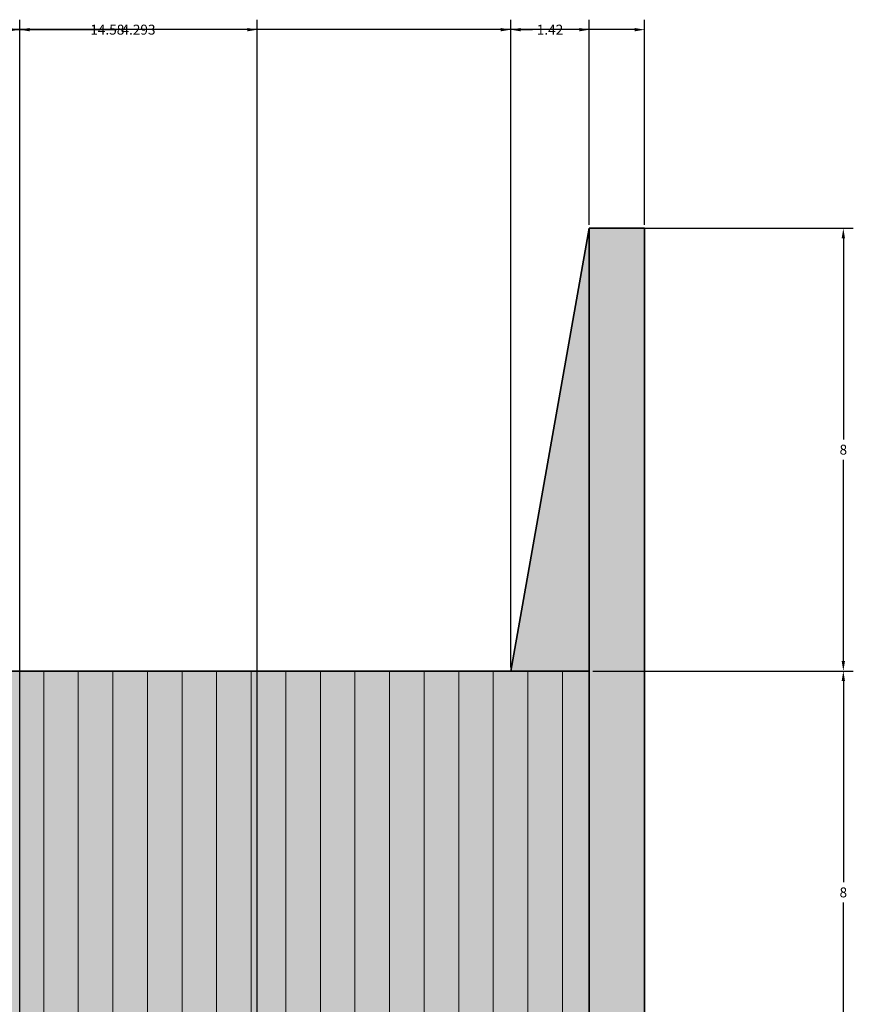
# Model space of a CAD drawing. Units: inches. Extents: x 18 to 59.8, y 2.7 to 81.2.
# Tile 9 of 9: x 44.6 to 59.6, y 63.4 to 81.2. Entities that reach past the tile are written whole.
import ezdxf

# ---------------------------------------------------------------- set-up
doc = ezdxf.new("R2010")
doc.units = ezdxf.units.IN
doc.header["$MEASUREMENT"] = 0
for name, color, linetype, lineweight in [('A-ANNO-DIMS', 2, 'Continuous', 18), ('A-ELEV', 7, 'Continuous', 35), ('A-ELEV-PATT', 8, 'Continuous', 13)]:
    doc.layers.add(name, color=color, linetype=linetype, lineweight=lineweight)
doc.styles.get("Standard").update_dxf_attribs({"font": 'arial.ttf'})
doc.dimstyles.get("Standard").update_dxf_attribs({"dimtxt": 0.18, "dimasz": 0.18, "dimexe": 0.18, "dimexo": 0.0625, "dimgap": 0.09, "dimtad": 0, "dimtih": 1, "dimtoh": 1, "dimdec": 1, "dimzin": 0, "dimdsep": 46, "dimlunit": 3, "dimtxsty": 'Standard', "dimcen": 0.09, "dimadec": 0, "dimazin": 0, "dimtfac": 1, "dimtdec": 1, "dimtofl": 0, "dimtmove": 0, "dimatfit": 3, "dimfxl": 1, "dimtolj": 1, "dimtzin": 0, "dimarcsym": 0})

# ---------------------------------------------------------------- blocks, each defined once
blk = doc.blocks.new('*D10')
at = {"layer": 'A-ANNO-DIMS', "color": 0, "lineweight": -2, "transparency": 16777216}
for p, q in [((21.859971, 77.503248), (21.859971, 81.210748)), ((55.859971, 77.503248), (55.859971, 81.210748)), ((22.039971, 81.03074799999999), (38.64147850341065, 81.03074799999999)), ((55.679971, 81.03074799999999), (39.07846349658936, 81.03074799999999))]:
    blk.add_line(p, q, dxfattribs=at)
at = {"layer": 'A-ANNO-DIMS', "color": 0, "transparency": 16777216}
for points in [[(22.039971, 81.060748), (22.039971, 81.00074799999999), (21.859971, 81.03074799999999)], [(55.679971, 81.060748), (55.679971, 81.00074799999999), (55.859971, 81.03074799999999)]]:
    blk.add_solid(points, dxfattribs=at)
at = {"layer": 'Defpoints', "color": 0, "transparency": 16777216}
for p in [(55.859971, 81.03074799999999), (21.859971, 77.44074799999999), (55.859971, 77.44074799999999)]:
    blk.add_point(p, dxfattribs=at)
at = {"layer": 'A-ANNO-DIMS', "color": 0, "transparency": 16777216, "insert": (38.859971, 81.03074799999999), "char_height": 0.18, "attachment_point": 5}
blk.add_mtext('\\A1;34', dxfattribs=at)
blk = doc.blocks.new('*D12')
at = {"layer": 'A-ANNO-DIMS', "color": 0, "lineweight": -2, "transparency": 16777216}
for p, q in [((38.859971, 69.503248), (38.859971, 81.210748)), ((53.440061, 69.503248), (53.440061, 81.210748)), ((39.039971, 81.03074799999999), (45.76459990177354, 81.03074799999999)), ((53.260061, 81.03074799999999), (46.53543209822646, 81.03074799999999))]:
    blk.add_line(p, q, dxfattribs=at)
at = {"layer": 'A-ANNO-DIMS', "color": 0, "transparency": 16777216}
for points in [[(39.039971, 81.060748), (39.039971, 81.00074799999999), (38.859971, 81.03074799999999)], [(53.260061, 81.060748), (53.260061, 81.00074799999999), (53.440061, 81.03074799999999)]]:
    blk.add_solid(points, dxfattribs=at)
at = {"layer": 'Defpoints', "color": 0, "transparency": 16777216}
for p in [(53.440061, 81.03074799999999), (38.859971, 69.440748), (53.440061, 69.440748)]:
    blk.add_point(p, dxfattribs=at)
at = {"layer": 'A-ANNO-DIMS', "color": 0, "transparency": 16777216, "insert": (46.150016, 81.03074799999999), "char_height": 0.18, "attachment_point": 5}
blk.add_mtext('\\A1;14.58', dxfattribs=at)
blk = doc.blocks.new('*D13')
at = {"layer": 'A-ANNO-DIMS', "color": 0, "lineweight": -2, "transparency": 16777216}
for p, q in [((53.440061, 69.503248), (53.440061, 81.210748)), ((54.859971, 77.503248), (54.859971, 81.210748)), ((53.620061, 81.03074799999999), (53.8356299154161, 81.03074799999999)), ((54.679971, 81.03074799999999), (54.4644020845839, 81.03074799999999))]:
    blk.add_line(p, q, dxfattribs=at)
at = {"layer": 'A-ANNO-DIMS', "color": 0, "transparency": 16777216}
for points in [[(53.620061, 81.060748), (53.620061, 81.00074799999999), (53.440061, 81.03074799999999)], [(54.679971, 81.060748), (54.679971, 81.00074799999999), (54.859971, 81.03074799999999)]]:
    blk.add_solid(points, dxfattribs=at)
at = {"layer": 'Defpoints', "color": 0, "transparency": 16777216}
for p in [(54.859971, 81.03074799999999), (54.859971, 77.44074799999999), (53.440061, 69.440748)]:
    blk.add_point(p, dxfattribs=at)
at = {"layer": 'A-ANNO-DIMS', "color": 0, "transparency": 16777216, "insert": (54.150016, 81.03074799999999), "char_height": 0.18, "attachment_point": 5}
blk.add_mtext('\\A1;1.42', dxfattribs=at)
blk = doc.blocks.new('*D21')
at = {"layer": 'A-ANNO-DIMS', "color": 0, "lineweight": -2, "transparency": 16777216}
for p, q in [((54.92247100000003, 69.44074800000001), (59.62997100000006, 69.44074800000001)), ((59.44997100000005, 69.26074800000002), (59.44997100000005, 65.62265113778993)), ((59.44997100000005, 61.62074800000002), (59.44997100000005, 65.25884486221013)), ((54.92247100000003, 61.44074800000002), (59.62997100000006, 61.44074800000002))]:
    blk.add_line(p, q, dxfattribs=at)
at = {"layer": 'A-ANNO-DIMS', "color": 0, "transparency": 16777216}
for points in [[(59.41997100000005, 69.26074800000002), (59.47997100000005, 69.26074800000002), (59.44997100000005, 69.44074800000001)], [(59.41997100000005, 61.62074800000002), (59.47997100000005, 61.62074800000002), (59.44997100000005, 61.44074800000002)]]:
    blk.add_solid(points, dxfattribs=at)
at = {"layer": 'Defpoints', "color": 0, "transparency": 16777216}
for p in [(54.85997100000003, 69.44074800000001), (59.44997100000005, 69.44074800000001), (54.85997100000003, 61.44074800000002)]:
    blk.add_point(p, dxfattribs=at)
at = {"layer": 'A-ANNO-DIMS', "color": 0, "transparency": 16777216, "insert": (59.44997100000006, 65.440748), "char_height": 0.18, "attachment_point": 5}
blk.add_mtext('\\A1;8', dxfattribs=at)
blk = doc.blocks.new('*D22')
at = {"layer": 'A-ANNO-DIMS', "color": 0, "lineweight": -2, "transparency": 16777216}
for p, q in [((54.92247100000003, 77.44074800000003), (59.62997100000006, 77.44074800000003)), ((59.44997100000005, 77.26074800000002), (59.44997100000005, 73.62265113778993)), ((59.44997100000005, 69.62074800000003), (59.44997100000005, 73.25884486221013)), ((54.92247100000003, 69.44074800000001), (59.62997100000006, 69.44074800000001))]:
    blk.add_line(p, q, dxfattribs=at)
at = {"layer": 'A-ANNO-DIMS', "color": 0, "transparency": 16777216}
for points in [[(59.41997100000005, 77.26074800000002), (59.47997100000005, 77.26074800000002), (59.44997100000005, 77.44074800000003)], [(59.41997100000005, 69.62074800000003), (59.47997100000005, 69.62074800000003), (59.44997100000005, 69.44074800000001)]]:
    blk.add_solid(points, dxfattribs=at)
at = {"layer": 'Defpoints', "color": 0, "transparency": 16777216}
for p in [(54.85997100000003, 77.44074800000003), (59.44997100000005, 77.44074800000003), (54.85997100000003, 69.44074800000001)]:
    blk.add_point(p, dxfattribs=at)
at = {"layer": 'A-ANNO-DIMS', "color": 0, "transparency": 16777216, "insert": (59.44997100000006, 73.440748), "char_height": 0.18, "attachment_point": 5}
blk.add_mtext('\\A1;8', dxfattribs=at)
blk = doc.blocks.new('*D51')
at = {"layer": 'A-ANNO-DIMS', "color": 0, "lineweight": -2, "transparency": 16777216}
for p, q in [((34.011642, 44.50324799999999), (34.011642, 81.210748)), ((48.859971, 43.503248), (48.859971, 81.210748)), ((34.191642, 81.03074799999999), (40.98046543587994, 81.03074799999999)), ((48.679971, 81.03074799999999), (41.89114756412005, 81.03074799999999))]:
    blk.add_line(p, q, dxfattribs=at)
at = {"layer": 'A-ANNO-DIMS', "color": 0, "transparency": 16777216}
for points in [[(34.191642, 81.060748), (34.191642, 81.00074799999999), (34.011642, 81.03074799999999)], [(48.679971, 81.060748), (48.679971, 81.00074799999999), (48.859971, 81.03074799999999)]]:
    blk.add_solid(points, dxfattribs=at)
at = {"layer": 'Defpoints', "color": 0, "transparency": 16777216}
for p in [(48.859971, 81.03074799999999), (34.011642, 44.440748), (48.859971, 43.440748)]:
    blk.add_point(p, dxfattribs=at)
at = {"layer": 'A-ANNO-DIMS', "color": 0, "transparency": 16777216, "insert": (41.43580649999999, 81.03074799999999), "char_height": 0.18, "attachment_point": 5}
blk.add_mtext('\\A1;14.848', dxfattribs=at)
blk = doc.blocks.new('*D62')
at = {"layer": 'A-ANNO-DIMS', "color": 0, "lineweight": -2, "transparency": 16777216}
for p, q in [((32.567078, 57.203248), (32.567078, 81.210748)), ((44.567078, 57.203248), (44.567078, 81.210748)), ((32.747078, 81.03074799999999), (38.35754866848568, 81.03074799999999)), ((44.387078, 81.03074799999999), (38.77660733151433, 81.03074799999999))]:
    blk.add_line(p, q, dxfattribs=at)
at = {"layer": 'A-ANNO-DIMS', "color": 0, "transparency": 16777216}
for points in [[(32.747078, 81.060748), (32.747078, 81.00074799999999), (32.567078, 81.03074799999999)], [(44.387078, 81.060748), (44.387078, 81.00074799999999), (44.567078, 81.03074799999999)]]:
    blk.add_solid(points, dxfattribs=at)
at = {"layer": 'Defpoints', "color": 0, "transparency": 16777216}
for p in [(44.567078, 81.03074799999999), (32.567078, 57.140748), (44.567078, 57.140748)]:
    blk.add_point(p, dxfattribs=at)
at = {"layer": 'A-ANNO-DIMS', "color": 0, "transparency": 16777216, "insert": (38.567078, 81.03074799999999), "char_height": 0.18, "attachment_point": 5}
blk.add_mtext('\\A1;12', dxfattribs=at)
blk = doc.blocks.new('*D63')
at = {"layer": 'A-ANNO-DIMS', "color": 0, "lineweight": -2, "transparency": 16777216}
for p, q in [((44.567078, 57.203248), (44.567078, 81.210748)), ((48.859971, 58.503248), (48.859971, 81.210748)), ((44.747078, 81.03074799999999), (46.31619844270123, 81.03074799999999)), ((48.679971, 81.03074799999999), (47.11085055729877, 81.03074799999999))]:
    blk.add_line(p, q, dxfattribs=at)
at = {"layer": 'A-ANNO-DIMS', "color": 0, "transparency": 16777216}
for points in [[(44.747078, 81.060748), (44.747078, 81.00074799999999), (44.567078, 81.03074799999999)], [(48.679971, 81.060748), (48.679971, 81.00074799999999), (48.859971, 81.03074799999999)]]:
    blk.add_solid(points, dxfattribs=at)
at = {"layer": 'Defpoints', "color": 0, "transparency": 16777216}
for p in [(48.859971, 81.03074799999999), (48.859971, 58.440748), (44.567078, 57.140748)]:
    blk.add_point(p, dxfattribs=at)
at = {"layer": 'A-ANNO-DIMS', "color": 0, "transparency": 16777216, "insert": (46.7135245, 81.03074799999999), "char_height": 0.18, "attachment_point": 5}
blk.add_mtext('\\A1;4.293', dxfattribs=at)

msp = doc.modelspace()

# ---------------------------------------------------------------- hatches: boundary and pattern name
at = {"layer": 'A-ELEV-PATT'}
h = msp.add_hatch(color=256, dxfattribs=at)
h.set_gradient(color1=(255, 255, 255), color2=(199, 200, 202))
h.paths.add_polyline_path([(38.85997087182833, 75.45212783007513, 0.4125526599533602), (36.85997087192615, 77.44074750583997), (21.85997087182832, 77.44074750583995), (21.85997087182832, 22.44074750583995), (22.85997087182833, 22.44074750583995), (48.85997087182833, 22.44074750583996), (48.85997087182833, 30.92342676155402, 0.4074472928332927), (48.33023903111634, 31.44074750583995), (30.40609029701442, 31.44074750583996, -0.7603989452129261), (34.01164157247843, 44.44074750583996), (47.85997087182832, 44.44074750583995, -0.4142135623730951), (48.85997087182833, 43.44074750583994), (48.85997087182833, 48.44074750583995, 0.4142135623730955), (47.85997087182832, 49.44074750583995), (32.23382408177119, 49.44074750583993, -0.2243141867862321), (27.84111392101349, 52.84266085519661, -0.8480128940945467), (38.85997087182833, 61.44074750583993)])
h.paths.add_polyline_path([(55.85997087182832, 77.44074750583995), (54.85997087182832, 77.44074750583997), (54.85997087182832, 22.24074750583996), (55.85997087182832, 22.24074750583995)])
h.paths.add_polyline_path([(54.85997087182832, 51.54074750583995), (53.44006084017791, 51.54074750583996), (53.44006084017792, 29.64074750583996), (54.85997087182832, 29.64074750583996)])
h.paths.add_polyline_path([(54.85997087182832, 61.44074750583993), (53.44006084017791, 57.44074750583993), (53.44006084017791, 51.64074750583996), (54.85997087182832, 51.64074750583996)])
h.paths.add_polyline_path([(54.85997087182832, 29.44074750583995), (54.47100875861361, 29.44074750583995), (54.47100875861361, 22.24074750583996), (54.85997087182832, 22.24074750583996)])
h.paths.add_polyline_path([(55.57447446325177, 22.24074750583995), (54.85997087182832, 22.24074750583996), (54.57447446325178, 22.24074750583996), (53.93466996146642, 21.792542566958), (54.58769880335594, 21.54947740208223)])
h.paths.add_polyline_path([(54.59913950424823, 21.54521903603421), (53.94430429933965, 21.78895655088426), (53.94430429933965, 18.44074750583995), (54.59913950424823, 18.44074750583995)])
h.paths.add_polyline_path([(53.94430429933965, 21.78895655088427), (53.93466996146642, 21.792542566958), (53.58162006229036, 21.54521903603422), (53.58162006229036, 18.44074750583995), (53.94430429933965, 18.44074750583994)])
h.paths.add_polyline_path([(53.36475139777029, 20.69276091189374), (52.89555240690669, 21.06460517556268), (52.89555240690669, 18.44074750583995), (53.3647513977703, 18.44074750583994)])
h.paths.add_polyline_path([(52.89555240690669, 21.06460517556268), (50.57752474318004, 19.44074750583995), (50.57752474318004, 18.44074750583995), (52.89555240690669, 18.44074750583995)])
h.paths.add_polyline_path([(53.58162006229036, 21.54521903603423), (52.89555240690668, 21.06460517556268), (53.3647513977703, 20.69276091189373), (53.58162006229036, 20.84468482967704)])
h.paths.add_polyline_path([(26.81093959479239, 19.44074750583995), (24.96715419074249, 20.84074750583995), (24.96715419074249, 18.44074750583995), (26.81093959479239, 18.44074750583995)])
h.paths.add_polyline_path([(24.96715419074249, 20.84074750583995), (24.41645576890079, 20.84268308307895), (24.41645576890079, 18.44074750583994), (24.96715419074249, 18.44074750583994)])
h.paths.add_polyline_path([(24.41645576890079, 20.84268308307895), (24.41645576890079, 21.25889692219009), (24.05877847081848, 21.5304839605815), (24.03006070560372, 21.51834150822755), (24.03006070560372, 18.44074750583995), (24.41645576890079, 18.44074750583995)])
h.paths.add_polyline_path([(24.03006070560372, 21.51834150822755), (23.41645576890078, 21.2588969221901), (23.41645576890078, 18.44074750583996), (24.03006070560372, 18.44074750583995)])
h.paths.add_polyline_path([(24.03006070560372, 21.51834150822755), (24.05877847081849, 21.53048396058151), (23.12336878669258, 22.24074750583995), (22.12336878669259, 22.24074750583996), (23.41645576890079, 21.2588969221901)])
h.paths.add_polyline_path([(24.41645576890079, 21.2588969221901), (24.41645576890079, 20.84268308307896), (24.96715419074249, 20.84074750583994)])
h.paths.add_polyline_path([(47.85997087182832, 18.44074750583995), (29.85997087182832, 18.44074750583995), (29.85997087182832, 6.440747505839951), (30.85997087182832, 6.440747505839937), (30.85997087182832, 17.44074750583995), (38.85997087182833, 17.44074750583995), (46.85997087182832, 17.44074750583995), (46.85997087182832, 6.440747505839937), (47.85997087182832, 6.440747505839958)])
h.paths.add_polyline_path([(54.57559250001032, 15.2149800477124), (54.57559250001032, 6.440747505839944), (55.85997087182832, 6.440747505839951), (55.85997087182832, 18.44074750583995), (47.85997087182832, 18.44074750583995), (47.85997087182832, 6.440747505839944), (49.14824210254597, 6.440747505839944), (49.14824210254597, 15.2149800477124, -1)])
h = msp.add_hatch(color=256, dxfattribs=at)
h.paths.add_polyline_path([(27.84111392101356, 52.84266085519647, -0.7443789445921651), (36.85997087182832, 61.44074750583993), (38.85997087182833, 61.44074750583993, 0.8480128940945556)])
h.paths.add_polyline_path([(47.85997087182832, 44.44074750583995), (34.01164157247843, 44.44074750583996, 0.7603989452129407), (30.40609029701462, 31.44074750583983, -0.7376245609052545), (34.01164157247731, 43.44074750583994), (47.85997087182831, 43.44074750583994, -0.4142135623730951), (48.85997087182832, 42.44074750583995), (48.85997087182833, 43.44074750583994, 0.4142135623730951)])
h.paths.add_polyline_path([(54.57559250001032, 15.2149800477124), (54.57559250001032, 6.440747505839951), (55.85997087182832, 6.440747505839951), (55.85997087182832, 18.44074750583995), (47.85997087182832, 18.44074750583995), (47.85997087182832, 6.440747505839944), (49.14824210254597, 6.440747505839944), (49.14824210254597, 15.2149800477124, -1)])
h.paths.add_polyline_path([(47.85997087182832, 18.44074750583995), (29.85997087182832, 18.44074750583995), (29.85997087182832, 6.440747505839958), (30.85997087182832, 6.440747505839951), (30.85997087182832, 17.44074750583995), (38.85997087182833, 17.44074750583995), (46.85997087182832, 17.44074750583995), (46.85997087182832, 6.440747505839944), (47.85997087182832, 6.440747505839951)])
h.paths.add_polyline_path([(55.85997087182832, 77.44074750583995), (54.85997087182832, 77.44074750583997), (54.85997087182833, 22.24074750583995), (55.85997087182832, 22.24074750583995)])
h = msp.add_hatch(color=256, dxfattribs=at)
h.set_gradient(color1=(147, 149, 152))
h.paths.add_polyline_path([(54.85997087182832, 77.44074750583995), (53.44006084017792, 69.44074750583995), (54.85997087182832, 69.44074750583995)])
h = msp.add_hatch(color=256, dxfattribs=at)
h.dxf.hatch_style = 1
h.paths.add_polyline_path([(54.85997087182832, 69.44074750583995), (38.85997087182833, 69.44074750583995), (38.85997087182833, 61.44074750583995), (54.85997087182832, 61.44074750583994)])
h.paths.add_polyline_path([(54.85997087182833, 61.44074750583994), (38.85997087182833, 61.44074750583995), (36.85997087182832, 61.44074750583993, 0.4434140223301819), (27.69861713021859, 58.44074750583995), (48.85997087182833, 58.44074750583995), (48.85997087182833, 57.44074750583994), (53.44006084017792, 57.44074750583995)])
h.paths.add_polyline_path([(37.49943513222304, 59.93991004599954), (37.49943513222304, 59.81982440572959, -2.410649922227508), (37.11866134610267, 59.81982440572959), (37.11866134610267, 59.93991004599954)], flags=16)
h.paths.add_polyline_path([(42.61253184194623, 59.80122867549901), (42.61253184194623, 59.92131431576897), (42.9933056280666, 59.92131431576897), (42.9933056280666, 59.80122867549901, -2.410649922227521)], flags=16)
h.paths.add_polyline_path([(49.59651616109447, 59.97095150496527), (49.59651616109447, 60.09103714523522), (49.97728994721485, 60.09103714523522), (49.97728994721485, 59.97095150496527, -2.410649922227521)], flags=16)
h.paths.add_polyline_path([(44.46707765301489, 57.04074750583994), (32.6670776530149, 57.04074750583994), (32.6670776530149, 56.04074750583993), (44.46707765301489, 56.04074750583993)])
h.paths.add_polyline_path([(47.85997087182831, 43.44074750583994), (46.85997087182832, 43.44074750583994), (34.0116415724774, 43.44074750583994, 0.2012982920418866), (29.34810857035394, 41.44074750583995), (47.85997087182831, 41.44074750583995, 1)])
h.paths.add_polyline_path([(36.55415719635351, 42.51454569609198), (36.55415719635351, 42.63463133636193), (36.93493098247388, 42.63463133636193), (36.93493098247388, 42.51454569609198, -2.410649922227513)], flags=16)
h.paths.add_polyline_path([(42.93899993637245, 42.54016758592221), (42.93899993637245, 42.66025322619216), (43.31977372249282, 42.66025322619216), (43.31977372249282, 42.54016758592221, -2.410649922227521)], flags=16)
h.paths.add_polyline_path([(54.47100875861361, 29.44074750583995), (48.85997087182833, 29.44074750583995), (48.85997087182833, 22.24074750583995), (54.47100875861361, 22.24074750583995)])
h.paths.add_polyline_path([(54.57447446325178, 22.24074750583996), (23.12336878669258, 22.24074750583996), (26.81093959479238, 19.44074750583996), (50.57752474318006, 19.44074750583996)])
h.paths.add_polyline_path([(54.57559250001032, 15.2149800477124, 1), (49.14824210254597, 15.2149800477124), (49.14824210254597, 6.440747505839958), (54.57559250001032, 6.440747505839965)])
h.paths.add_polyline_path([(49.83226884926398, 12.6020427608384), (49.83226884926398, 9.122455521673542), (49.66565363924473, 9.122455521673537), (49.66565363924473, 12.6020427608384)], flags=16)
h = msp.add_hatch(dxfattribs=at)
h.set_pattern_fill('ANSI31', color=256, scale=5, angle=45, style=0)
h.set_pattern_definition([(90, (0, 0), (-0.6250000000000001, 0), [])])
h.paths.add_polyline_path([(54.85997087182832, 69.44074750583995), (38.85997087182833, 69.44074750583995), (38.85997087182833, 61.44074750583995), (54.85997087182832, 61.44074750583994)])
h.paths.add_polyline_path([(54.85997087182833, 61.44074750583994), (38.85997087182833, 61.44074750583995), (36.85997087182832, 61.44074750583993, 0.4434140223301819), (27.69861713021859, 58.44074750583995), (48.85997087182833, 58.44074750583995), (48.85997087182833, 57.44074750583994), (53.44006084017792, 57.44074750583995)])
h.paths.add_polyline_path([(37.16613704638868, 59.85769359025997), (37.11866134610267, 59.85769359025997), (37.11866134610267, 59.93991004599954), (37.49943513222304, 59.93991004599954), (37.49943513222304, 59.85769359025997), (37.45195943193702, 59.85769359025997, -3.476462016968403)], flags=16)
h.paths.add_polyline_path([(42.66000754223224, 59.8390978600294), (42.61253184194623, 59.8390978600294), (42.61253184194623, 59.92131431576897), (42.9933056280666, 59.92131431576897), (42.9933056280666, 59.8390978600294), (42.94582992778058, 59.8390978600294, -3.47646201696846)], flags=16)
h.paths.add_polyline_path([(49.64399186138049, 60.00882068949565), (49.59651616109447, 60.00882068949565), (49.59651616109447, 60.09103714523522), (49.97728994721485, 60.09103714523522), (49.97728994721485, 60.00882068949565), (49.92981424692883, 60.00882068949565, -3.476462016968434)], flags=16)
h.paths.add_polyline_path([(44.46707765301489, 57.04074750583994), (32.6670776530149, 57.04074750583994), (32.6670776530149, 56.04074750583993), (44.46707765301489, 56.04074750583993)])
h.paths.add_polyline_path([(47.85997087182831, 43.44074750583994), (46.85997087182832, 43.44074750583994), (34.0116415724774, 43.44074750583994, 0.2012982920418866), (29.34810857035394, 41.44074750583995), (47.85997087182831, 41.44074750583995, 1)])
h.paths.add_polyline_path([(36.60163289663952, 42.55241488062237), (36.55415719635351, 42.55241488062236), (36.55415719635351, 42.63463133636193), (36.93493098247388, 42.63463133636193), (36.93493098247388, 42.55241488062236), (36.88745528218787, 42.55241488062236, -3.476462016968307)], flags=16)
h.paths.add_polyline_path([(42.98647563665846, 42.5780367704526), (42.93899993637245, 42.5780367704526), (42.93899993637245, 42.66025322619216), (43.31977372249282, 42.66025322619216), (43.31977372249282, 42.57803677045259), (43.2722980222068, 42.57803677045259, -3.476462016968351)], flags=16)
h.paths.add_polyline_path([(54.47100875861361, 29.44074750583995), (48.85997087182833, 29.44074750583995), (48.85997087182833, 22.24074750583995), (54.47100875861361, 22.24074750583994)])
h.paths.add_polyline_path([(54.57447446325179, 22.24074750583995), (23.12336878669258, 22.24074750583995), (26.81093959479238, 19.44074750583996), (50.57752474318005, 19.44074750583996)])
h.paths.add_polyline_path([(54.57559250001032, 15.2149800477124, 1), (49.14824210254597, 15.2149800477124), (49.14824210254597, 6.440747505839958), (54.57559250001032, 6.440747505839944)])
h.paths.add_polyline_path([(49.83226884926398, 9.122455521673542), (49.66565363924473, 9.122455521673537), (49.66565363924473, 12.60204276083839), (49.83226884926398, 12.6020427608384)], flags=16)

# ---------------------------------------------------------------- linework, layer by layer
at = {"layer": 'A-ELEV'}
for p, q in [((54.85997087182832, 77.44074750583995), (53.44006084017792, 69.44074750583995)), ((54.85997087182833, 22.24074750583995), (54.85997087182832, 77.44074750583995)), ((55.85997087182832, 77.44074750583995), (54.85997087182832, 77.44074750583997)), ((55.85997087182832, 77.44074750583994), (55.85997087182832, 22.24074750583995)), ((54.85997087182833, 69.44074750583995), (38.85997087182833, 69.44074750583995))]:
    msp.add_line(p, q, dxfattribs=at)

# ---------------------------------------------------------------- dimensions: what is measured, and where the dimension line sits
at = {"layer": 'A-ANNO-DIMS'}
for base, p1, p2, override, picture, middle in [((55.859971, 81.03074799999999), (21.859971, 77.44074799999999), (55.859971, 77.44074799999999), {"dimdec": 0, "dimlfac": 1, "dimrnd": 0, "dimzin": 0, "dimdsep": 46, "dimlunit": 2}, '*D10', (38.859971, 81.03074799999999)), ((44.567078, 81.03074799999999), (32.567078, 57.140748), (44.567078, 57.140748), {"dimdec": 0, "dimlfac": 1, "dimrnd": 0, "dimzin": 0, "dimdsep": 46, "dimlunit": 2}, '*D62', (38.567078, 81.03074799999999)), ((48.859971, 81.03074799999999), (34.011642, 44.440748), (48.859971, 43.440748), {"dimdec": 3, "dimlfac": 1, "dimrnd": 0, "dimzin": 0, "dimdsep": 46, "dimlunit": 2}, '*D51', (41.43580649999999, 81.03074799999999)), ((53.440061, 81.03074799999999), (38.859971, 69.440748), (53.440061, 69.440748), {"dimdec": 2, "dimlfac": 1, "dimrnd": 0, "dimzin": 0, "dimdsep": 46, "dimlunit": 2}, '*D12', (46.150016, 81.03074799999999)), ((48.859971, 81.03074799999999), (44.567078, 57.140748), (48.859971, 58.440748), {"dimdec": 3, "dimlfac": 1, "dimrnd": 0, "dimzin": 0, "dimdsep": 46, "dimlunit": 2}, '*D63', (46.7135245, 81.03074799999999)), ((54.859971, 81.03074799999999), (53.440061, 69.440748), (54.859971, 77.44074799999999), {"dimdec": 2, "dimlfac": 1, "dimrnd": 0, "dimzin": 0, "dimdsep": 46, "dimlunit": 2}, '*D13', (54.150016, 81.03074799999999))]:
    dim = msp.add_linear_dim(base=base, p1=p1, p2=p2, dimstyle='Standard', override=override, dxfattribs=at)
    dim.commit()
    dim.dimension.update_dxf_attribs({"geometry": picture, "text_midpoint": middle})
for base, p1, p2, picture, middle in [((59.44997100000005, 77.44074800000003), (54.859971, 69.440748), (54.859971, 77.44074799999999), '*D22', (59.44997100000006, 73.440748)), ((59.44997100000005, 69.44074800000001), (54.859971, 61.440748), (54.859971, 69.440748), '*D21', (59.44997100000006, 65.440748))]:
    dim = msp.add_linear_dim(base=base, p1=p1, p2=p2, angle=90, dimstyle='Standard', override={"dimdec": 0, "dimlfac": 1, "dimrnd": 0, "dimzin": 0, "dimdsep": 46, "dimlunit": 2}, dxfattribs=at)
    dim.commit()
    dim.dimension.update_dxf_attribs({"geometry": picture, "text_midpoint": middle})

doc.saveas('drawing.dxf')
